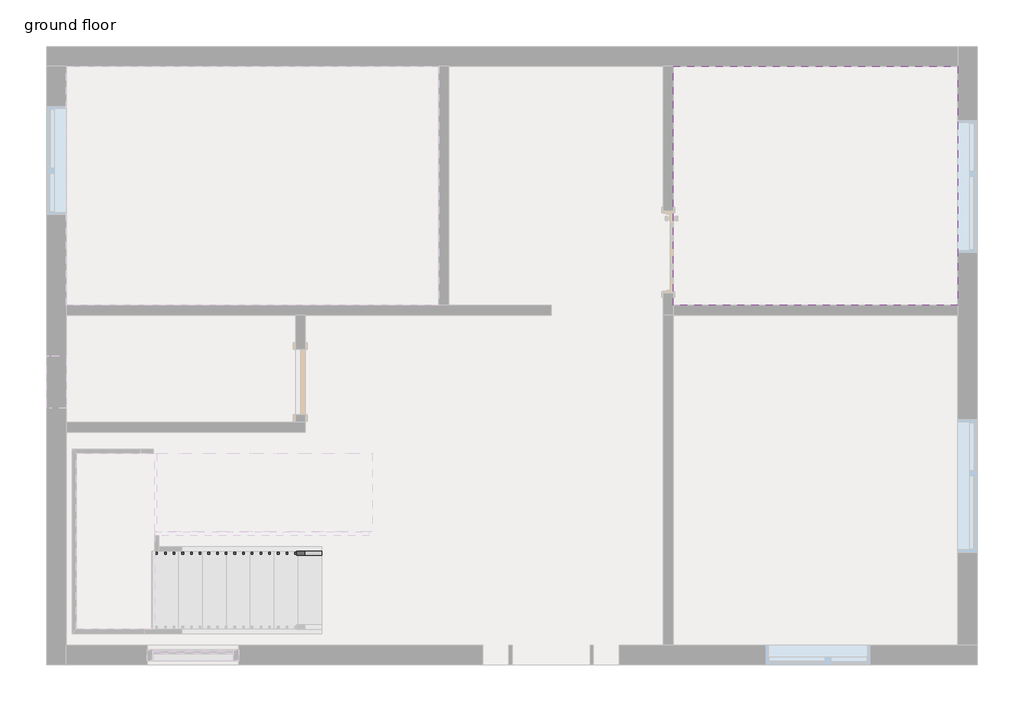
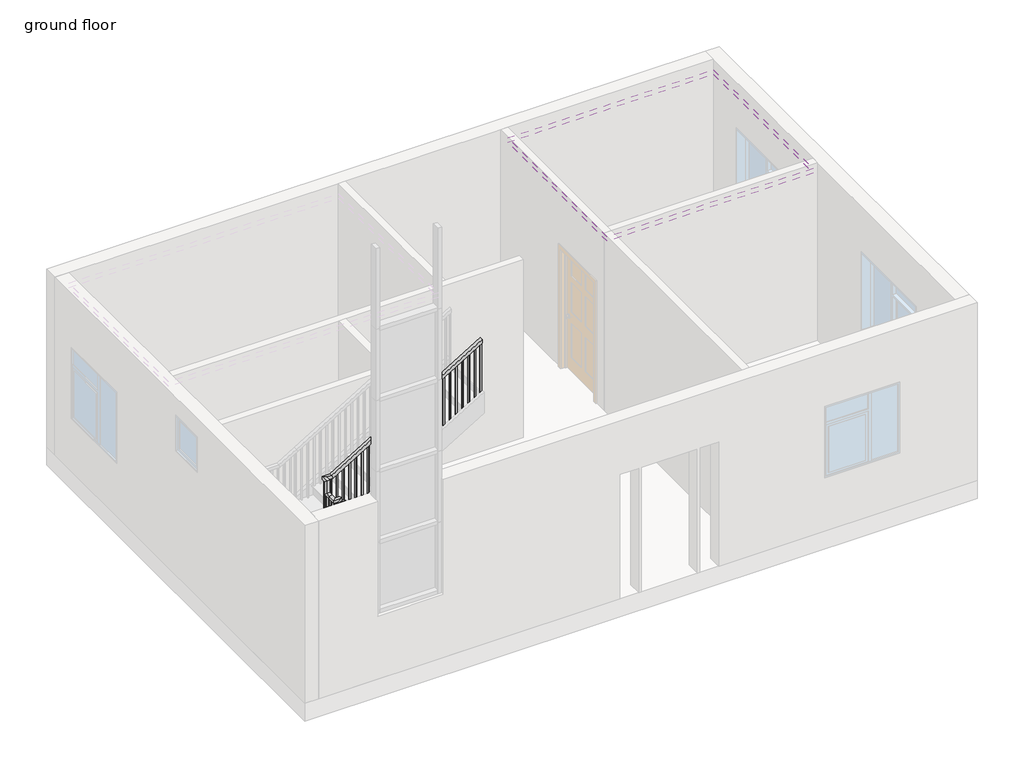
# One storey, part 2 of 3: 2 coverings, 1 railing.
"""IFC4 building model written with IfcOpenShell, lengths in millimetres."""

from ifc_helpers import new_model, si_unit, frame, origin, place, context, project, spatial, polyline, outline, extrude, faceted_brep, element, save

model = new_model("IFC4")

# Units and contexts
model_context = context("Model", 3, world=origin())
ifc_project = project(units=[si_unit("LENGTHUNIT", "METRE", prefix="MILLI")], contexts=[model_context])

# Site, building, storey
site = spatial("IfcSite", under=ifc_project)
building = spatial("IfcBuilding", under=site)
storey = spatial("IfcBuildingStorey", under=building, Name="ground floor", Elevation=304.8)

# Coverings
placement = place(None, origin())
element("IfcCovering", 1, ObjectType="METAL WHITE CEILING", at=placement, inside=storey, context=model_context, shape_type="SweptSolid", body=[
    extrude(outline(polyline([(-8505.3777023, 3436.0179075), (-8505.3777023, 6236.3679075), (-5171.6277023, 6236.3679075), (-5171.6277023, 3436.0179075), (-8505.3777023, 3436.0179075)])), frame((0.0, 0.0, 3175.0), z_axis=(0.0, 0.0, 1.0), x_axis=(1.0, 0.0, 0.0)), (0.0, 0.0, 1.0), 107.95),
])
element("IfcCovering", 2, ObjectType="METAL WHITE CEILING", at=placement, inside=storey, context=model_context, shape_type="SweptSolid", body=[
    extrude(outline(polyline([(-5171.6277023, 6236.3679075), (-5171.6277023, 3436.0179075), (-8505.3777023, 3436.0179075), (-8505.3777023, 6236.3679075), (-5171.6277023, 6236.3679075)]), holes=[polyline([(-5476.4277023, 5931.5679075), (-8200.5777023, 5931.5679075), (-8200.5777023, 3740.8179075), (-5476.4277023, 3740.8179075), (-5476.4277023, 5931.5679075)])]), frame((0.0, 0.0, 3098.8), z_axis=(0.0, 0.0, 1.0), x_axis=(1.0, 0.0, 0.0)), (0.0, 0.0, 1.0), 107.95),
    extrude(outline(polyline([(-7575.2115209, 5626.7679075), (-7575.2115209, 4045.6179075), (-7880.0115209, 4045.6179075), (-7880.0115209, 5626.7679075), (-7575.2115209, 5626.7679075)])), frame((0.0, 0.0, 3098.8), z_axis=(0.0, 0.0, 1.0), x_axis=(1.0, 0.0, 0.0)), (0.0, 0.0, 1.0), 107.95),
    extrude(outline(polyline([(-6965.6115209, 5626.7679075), (-6965.6115209, 4045.6179075), (-7270.4115209, 4045.6179075), (-7270.4115209, 5626.7679075), (-6965.6115209, 5626.7679075)])), frame((0.0, 0.0, 3098.8), z_axis=(0.0, 0.0, 1.0), x_axis=(1.0, 0.0, 0.0)), (0.0, 0.0, 1.0), 107.95),
    extrude(outline(polyline([(-6356.0115209, 5626.7679075), (-6356.0115209, 4045.6179075), (-6660.8115209, 4045.6179075), (-6660.8115209, 5626.7679075), (-6356.0115209, 5626.7679075)])), frame((0.0, 0.0, 3098.8), z_axis=(0.0, 0.0, 1.0), x_axis=(1.0, 0.0, 0.0)), (0.0, 0.0, 1.0), 107.95),
    extrude(outline(polyline([(-5746.4115209, 5626.7679075), (-5746.4115209, 4045.6179075), (-6051.2115209, 4045.6179075), (-6051.2115209, 5626.7679075), (-5746.4115209, 5626.7679075)])), frame((0.0, 0.0, 3098.8), z_axis=(0.0, 0.0, 1.0), x_axis=(1.0, 0.0, 0.0)), (0.0, 0.0, 1.0), 107.95),
])

# Railing
element("IfcRailing", 3, ObjectType="Handrail - Rectangular", at=placement, inside=storey, context=model_context, shape_type="SolidModel", body=[
    faceted_brep([(-12620.1777023, 508.6679075, 1388.5333333), (-12620.1777023, 508.6679075, 1329.1318731), (-12620.1777023, 559.4679075, 1329.1318731), (-12620.1777023, 559.4679075, 1388.5333333), (-14499.7777023, 508.6679075, 2527.6848485), (-14550.5777023, 508.6679075, 2499.071267), (-14550.5777023, 559.4679075, 2499.071267), (-14499.7777023, 559.4679075, 2527.6848485), (-14499.7777023, 508.6679075, 2573.8666667), (-14550.5777023, 508.6679075, 2523.0666667), (-14550.5777023, 559.4679075, 2523.0666667), (-14499.7777023, 559.4679075, 2573.8666667), (-14626.7777023, 508.6679075, 2573.8666667), (-14626.7777023, 508.6679075, 2523.0666667), (-14575.9777023, 559.4679075, 2523.0666667), (-14575.9777023, 559.4679075, 2573.8666667), (-14626.7777023, 635.6679075, 2573.8666667), (-14626.7777023, 635.6679075, 2523.0666667), (-14575.9777023, 635.6679075, 2523.0666667), (-14575.9777023, 635.6679075, 2573.8666667), (-14626.7777023, 711.8679075, 2573.8666667), (-14626.7777023, 762.6679075, 2523.0666667), (-14575.9777023, 762.6679075, 2523.0666667), (-14575.9777023, 711.8679075, 2573.8666667), (-14626.7777023, 711.8679075, 2789.3818182), (-14626.7777023, 762.6679075, 2738.5818182), (-14575.9777023, 762.6679075, 2738.5818182), (-14575.9777023, 711.8679075, 2789.3818182), (-14626.7777023, 838.8679075, 2789.3818182), (-14626.7777023, 838.8679075, 2738.5818182), (-14575.9777023, 788.0679075, 2738.5818182), (-14575.9777023, 788.0679075, 2789.3818182), (-14499.7777023, 838.8679075, 2789.3818182), (-14485.5852929, 838.8679075, 2738.5818182), (-14485.5852929, 788.0679075, 2738.5818182), (-14499.7777023, 788.0679075, 2789.3818182), (-12061.3777023, 838.8679075, 4267.2), (-12061.3777023, 788.0679075, 4267.2), (-12061.3777023, 788.0679075, 4207.7985397), (-12061.3777023, 838.8679075, 4207.7985397)], [[[0, 1, 2, 3]], [[1, 0, 4, 5]], [[2, 1, 5, 6]], [[3, 2, 6, 7]], [[0, 3, 7, 4]], [[5, 4, 8, 9]], [[6, 5, 9, 10]], [[7, 6, 10, 11]], [[4, 7, 11, 8]], [[9, 8, 12, 13]], [[10, 9, 13, 14]], [[11, 10, 14, 15]], [[8, 11, 15, 12]], [[13, 12, 16, 17]], [[14, 13, 17, 18]], [[15, 14, 18, 19]], [[12, 15, 19, 16]], [[17, 16, 20, 21]], [[18, 17, 21, 22]], [[19, 18, 22, 23]], [[16, 19, 23, 20]], [[21, 20, 24, 25]], [[22, 21, 25, 26]], [[23, 22, 26, 27]], [[20, 23, 27, 24]], [[25, 24, 28, 29]], [[26, 25, 29, 30]], [[27, 26, 30, 31]], [[24, 27, 31, 28]], [[29, 28, 32, 33]], [[30, 29, 33, 34]], [[31, 30, 34, 35]], [[28, 31, 35, 32]], [[36, 37, 38, 39]], [[33, 32, 36, 39]], [[34, 33, 39, 38]], [[35, 34, 38, 37]], [[32, 35, 37, 36]]]),
    extrude(outline(polyline([(4151.9955094, -12153.4527023), (4140.4500549, -12172.5027023), (3183.4666667, -12172.5027023), (3183.4666667, -12153.4527023), (4151.9955094, -12153.4527023)])), frame((0.0, 803.9429075, 0.0), z_axis=(0.0, 1.0, 0.0), x_axis=(0.0, 0.0, 1.0)), (0.0, 0.0, 1.0), 19.05),
    extrude(outline(polyline([(4090.4197519, -12255.0527023), (4078.8742973, -12274.1027023), (3183.4666667, -12274.1027023), (3183.4666667, -12255.0527023), (4090.4197519, -12255.0527023)])), frame((0.0, 803.9429075, 0.0), z_axis=(0.0, 1.0, 0.0), x_axis=(0.0, 0.0, 1.0)), (0.0, 0.0, 1.0), 19.05),
    extrude(outline(polyline([(4028.8439943, -12356.6527023), (4017.2985397, -12375.7027023), (3014.1333333, -12375.7027023), (3014.1333333, -12356.6527023), (4028.8439943, -12356.6527023)])), frame((0.0, 803.9429075, 0.0), z_axis=(0.0, 1.0, 0.0), x_axis=(0.0, 0.0, 1.0)), (0.0, 0.0, 1.0), 19.05),
    extrude(outline(polyline([(3967.2682367, -12458.2527023), (3955.7227822, -12477.3027023), (3014.1333333, -12477.3027023), (3014.1333333, -12458.2527023), (3967.2682367, -12458.2527023)])), frame((0.0, 803.9429075, 0.0), z_axis=(0.0, 1.0, 0.0), x_axis=(0.0, 0.0, 1.0)), (0.0, 0.0, 1.0), 19.05),
    extrude(outline(polyline([(3905.6924791, -12559.8527023), (3894.1470246, -12578.9027023), (3014.1333333, -12578.9027023), (3014.1333333, -12559.8527023), (3905.6924791, -12559.8527023)])), frame((0.0, 803.9429075, 0.0), z_axis=(0.0, 1.0, 0.0), x_axis=(0.0, 0.0, 1.0)), (0.0, 0.0, 1.0), 19.05),
    extrude(outline(polyline([(3844.1167216, -12661.4527023), (3832.571267, -12680.5027023), (2844.8, -12680.5027023), (2844.8, -12661.4527023), (3844.1167216, -12661.4527023)])), frame((0.0, 803.9429075, 0.0), z_axis=(0.0, 1.0, 0.0), x_axis=(0.0, 0.0, 1.0)), (0.0, 0.0, 1.0), 19.05),
    extrude(outline(polyline([(3782.540964, -12763.0527023), (3770.9955094, -12782.1027023), (2844.8, -12782.1027023), (2844.8, -12763.0527023), (3782.540964, -12763.0527023)])), frame((0.0, 803.9429075, 0.0), z_axis=(0.0, 1.0, 0.0), x_axis=(0.0, 0.0, 1.0)), (0.0, 0.0, 1.0), 19.05),
    extrude(outline(polyline([(3720.9652064, -12864.6527023), (3709.4197519, -12883.7027023), (2844.8, -12883.7027023), (2844.8, -12864.6527023), (3720.9652064, -12864.6527023)])), frame((0.0, 803.9429075, 0.0), z_axis=(0.0, 1.0, 0.0), x_axis=(0.0, 0.0, 1.0)), (0.0, 0.0, 1.0), 19.05),
    extrude(outline(polyline([(3659.3894488, -12966.2527023), (3647.8439943, -12985.3027023), (2675.4666667, -12985.3027023), (2675.4666667, -12966.2527023), (3659.3894488, -12966.2527023)])), frame((0.0, 803.9429075, 0.0), z_axis=(0.0, 1.0, 0.0), x_axis=(0.0, 0.0, 1.0)), (0.0, 0.0, 1.0), 19.05),
    extrude(outline(polyline([(3597.8136913, -13067.8527023), (3586.2682367, -13086.9027023), (2675.4666667, -13086.9027023), (2675.4666667, -13067.8527023), (3597.8136913, -13067.8527023)])), frame((0.0, 803.9429075, 0.0), z_axis=(0.0, 1.0, 0.0), x_axis=(0.0, 0.0, 1.0)), (0.0, 0.0, 1.0), 19.05),
    extrude(outline(polyline([(3536.2379337, -13169.4527023), (3524.6924791, -13188.5027023), (2675.4666667, -13188.5027023), (2675.4666667, -13169.4527023), (3536.2379337, -13169.4527023)])), frame((0.0, 803.9429075, 0.0), z_axis=(0.0, 1.0, 0.0), x_axis=(0.0, 0.0, 1.0)), (0.0, 0.0, 1.0), 19.05),
    extrude(outline(polyline([(3474.6621761, -13271.0527023), (3463.1167216, -13290.1027023), (2506.1333333, -13290.1027023), (2506.1333333, -13271.0527023), (3474.6621761, -13271.0527023)])), frame((0.0, 803.9429075, 0.0), z_axis=(0.0, 1.0, 0.0), x_axis=(0.0, 0.0, 1.0)), (0.0, 0.0, 1.0), 19.05),
    extrude(outline(polyline([(3413.0864185, -13372.6527023), (3401.540964, -13391.7027023), (2506.1333333, -13391.7027023), (2506.1333333, -13372.6527023), (3413.0864185, -13372.6527023)])), frame((0.0, 803.9429075, 0.0), z_axis=(0.0, 1.0, 0.0), x_axis=(0.0, 0.0, 1.0)), (0.0, 0.0, 1.0), 19.05),
    extrude(outline(polyline([(3351.510661, -13474.2527023), (3339.9652064, -13493.3027023), (2336.8, -13493.3027023), (2336.8, -13474.2527023), (3351.510661, -13474.2527023)])), frame((0.0, 803.9429075, 0.0), z_axis=(0.0, 1.0, 0.0), x_axis=(0.0, 0.0, 1.0)), (0.0, 0.0, 1.0), 19.05),
    extrude(outline(polyline([(3289.9349034, -13575.8527023), (3278.3894488, -13594.9027023), (2336.8, -13594.9027023), (2336.8, -13575.8527023), (3289.9349034, -13575.8527023)])), frame((0.0, 803.9429075, 0.0), z_axis=(0.0, 1.0, 0.0), x_axis=(0.0, 0.0, 1.0)), (0.0, 0.0, 1.0), 19.05),
    extrude(outline(polyline([(3228.3591458, -13677.4527023), (3216.8136913, -13696.5027023), (2336.8, -13696.5027023), (2336.8, -13677.4527023), (3228.3591458, -13677.4527023)])), frame((0.0, 803.9429075, 0.0), z_axis=(0.0, 1.0, 0.0), x_axis=(0.0, 0.0, 1.0)), (0.0, 0.0, 1.0), 19.05),
    extrude(outline(polyline([(3166.7833882, -13779.0527023), (3155.2379337, -13798.1027023), (2167.4666667, -13798.1027023), (2167.4666667, -13779.0527023), (3166.7833882, -13779.0527023)])), frame((0.0, 803.9429075, 0.0), z_axis=(0.0, 1.0, 0.0), x_axis=(0.0, 0.0, 1.0)), (0.0, 0.0, 1.0), 19.05),
    extrude(outline(polyline([(3105.2076307, -13880.6527023), (3093.6621761, -13899.7027023), (2167.4666667, -13899.7027023), (2167.4666667, -13880.6527023), (3105.2076307, -13880.6527023)])), frame((0.0, 803.9429075, 0.0), z_axis=(0.0, 1.0, 0.0), x_axis=(0.0, 0.0, 1.0)), (0.0, 0.0, 1.0), 19.05),
    extrude(outline(polyline([(3043.6318731, -13982.2527023), (3032.0864185, -14001.3027023), (2167.4666667, -14001.3027023), (2167.4666667, -13982.2527023), (3043.6318731, -13982.2527023)])), frame((0.0, 803.9429075, 0.0), z_axis=(0.0, 1.0, 0.0), x_axis=(0.0, 0.0, 1.0)), (0.0, 0.0, 1.0), 19.05),
    extrude(outline(polyline([(2982.0561155, -14083.8527023), (2970.510661, -14102.9027023), (1998.1333333, -14102.9027023), (1998.1333333, -14083.8527023), (2982.0561155, -14083.8527023)])), frame((0.0, 803.9429075, 0.0), z_axis=(0.0, 1.0, 0.0), x_axis=(0.0, 0.0, 1.0)), (0.0, 0.0, 1.0), 19.05),
    extrude(outline(polyline([(2920.4803579, -14185.4527023), (2908.9349034, -14204.5027023), (1998.1333333, -14204.5027023), (1998.1333333, -14185.4527023), (2920.4803579, -14185.4527023)])), frame((0.0, 803.9429075, 0.0), z_axis=(0.0, 1.0, 0.0), x_axis=(0.0, 0.0, 1.0)), (0.0, 0.0, 1.0), 19.05),
    extrude(outline(polyline([(2858.9046004, -14287.0527023), (2847.3591458, -14306.1027023), (1998.1333333, -14306.1027023), (1998.1333333, -14287.0527023), (2858.9046004, -14287.0527023)])), frame((0.0, 803.9429075, 0.0), z_axis=(0.0, 1.0, 0.0), x_axis=(0.0, 0.0, 1.0)), (0.0, 0.0, 1.0), 19.05),
    extrude(outline(polyline([(2797.3288428, -14388.6527023), (2785.7833882, -14407.7027023), (1828.8, -14407.7027023), (1828.8, -14388.6527023), (2797.3288428, -14388.6527023)])), frame((0.0, 803.9429075, 0.0), z_axis=(0.0, 1.0, 0.0), x_axis=(0.0, 0.0, 1.0)), (0.0, 0.0, 1.0), 19.05),
    extrude(outline(polyline([(2735.7530852, -14490.2527023), (2724.2076307, -14509.3027023), (1828.8, -14509.3027023), (1828.8, -14490.2527023), (2735.7530852, -14490.2527023)])), frame((0.0, 803.9429075, 0.0), z_axis=(0.0, 1.0, 0.0), x_axis=(0.0, 0.0, 1.0)), (0.0, 0.0, 1.0), 19.05),
    extrude(outline(polyline([(-14591.8527023, 727.7429075), (-14610.9027023, 727.7429075), (-14610.9027023, 746.7929075), (-14591.8527023, 746.7929075), (-14591.8527023, 727.7429075)])), frame((0.0, 0.0, 1659.4666667), z_axis=(0.0, 0.0, 1.0), x_axis=(1.0, 0.0, 0.0)), (0.0, 0.0, 1.0), 1079.1151515),
    extrude(outline(polyline([(-14591.8527023, 626.1429075), (-14610.9027023, 626.1429075), (-14610.9027023, 645.1929075), (-14591.8527023, 645.1929075), (-14591.8527023, 626.1429075)])), frame((0.0, 0.0, 1659.4666667), z_axis=(0.0, 0.0, 1.0), x_axis=(1.0, 0.0, 0.0)), (0.0, 0.0, 1.0), 863.6),
    extrude(outline(polyline([(-14541.0527023, 543.5929075), (-14541.0527023, 524.5429075), (-14560.1027023, 524.5429075), (-14560.1027023, 543.5929075), (-14541.0527023, 543.5929075)])), frame((0.0, 0.0, 1490.1333333), z_axis=(0.0, 0.0, 1.0), x_axis=(1.0, 0.0, 0.0)), (0.0, 0.0, 1.0), 1032.9333333),
    extrude(outline(polyline([(2431.7227822, -14439.4527023), (2443.2682367, -14458.5027023), (1490.1333333, -14458.5027023), (1490.1333333, -14439.4527023), (2431.7227822, -14439.4527023)])), frame((0.0, 524.5429075, 0.0), z_axis=(0.0, 1.0, 0.0), x_axis=(0.0, 0.0, 1.0)), (0.0, 0.0, 1.0), 19.05),
    extrude(outline(polyline([(2370.1470246, -14337.8527023), (2381.6924791, -14356.9027023), (1490.1333333, -14356.9027023), (1490.1333333, -14337.8527023), (2370.1470246, -14337.8527023)])), frame((0.0, 524.5429075, 0.0), z_axis=(0.0, 1.0, 0.0), x_axis=(0.0, 0.0, 1.0)), (0.0, 0.0, 1.0), 19.05),
    extrude(outline(polyline([(2308.571267, -14236.2527023), (2320.1167216, -14255.3027023), (1320.8, -14255.3027023), (1320.8, -14236.2527023), (2308.571267, -14236.2527023)])), frame((0.0, 524.5429075, 0.0), z_axis=(0.0, 1.0, 0.0), x_axis=(0.0, 0.0, 1.0)), (0.0, 0.0, 1.0), 19.05),
    extrude(outline(polyline([(2246.9955094, -14134.6527023), (2258.540964, -14153.7027023), (1320.8, -14153.7027023), (1320.8, -14134.6527023), (2246.9955094, -14134.6527023)])), frame((0.0, 524.5429075, 0.0), z_axis=(0.0, 1.0, 0.0), x_axis=(0.0, 0.0, 1.0)), (0.0, 0.0, 1.0), 19.05),
    extrude(outline(polyline([(2185.4197519, -14033.0527023), (2196.9652064, -14052.1027023), (1320.8, -14052.1027023), (1320.8, -14033.0527023), (2185.4197519, -14033.0527023)])), frame((0.0, 524.5429075, 0.0), z_axis=(0.0, 1.0, 0.0), x_axis=(0.0, 0.0, 1.0)), (0.0, 0.0, 1.0), 19.05),
    extrude(outline(polyline([(2123.8439943, -13931.4527023), (2135.3894488, -13950.5027023), (1151.4666667, -13950.5027023), (1151.4666667, -13931.4527023), (2123.8439943, -13931.4527023)])), frame((0.0, 524.5429075, 0.0), z_axis=(0.0, 1.0, 0.0), x_axis=(0.0, 0.0, 1.0)), (0.0, 0.0, 1.0), 19.05),
    extrude(outline(polyline([(2062.2682367, -13829.8527023), (2073.8136913, -13848.9027023), (1151.4666667, -13848.9027023), (1151.4666667, -13829.8527023), (2062.2682367, -13829.8527023)])), frame((0.0, 524.5429075, 0.0), z_axis=(0.0, 1.0, 0.0), x_axis=(0.0, 0.0, 1.0)), (0.0, 0.0, 1.0), 19.05),
    extrude(outline(polyline([(2000.6924791, -13728.2527023), (2012.2379337, -13747.3027023), (1151.4666667, -13747.3027023), (1151.4666667, -13728.2527023), (2000.6924791, -13728.2527023)])), frame((0.0, 524.5429075, 0.0), z_axis=(0.0, 1.0, 0.0), x_axis=(0.0, 0.0, 1.0)), (0.0, 0.0, 1.0), 19.05),
    extrude(outline(polyline([(1939.1167216, -13626.6527023), (1950.6621761, -13645.7027023), (982.1333333, -13645.7027023), (982.1333333, -13626.6527023), (1939.1167216, -13626.6527023)])), frame((0.0, 524.5429075, 0.0), z_axis=(0.0, 1.0, 0.0), x_axis=(0.0, 0.0, 1.0)), (0.0, 0.0, 1.0), 19.05),
    extrude(outline(polyline([(1877.540964, -13525.0527023), (1889.0864185, -13544.1027023), (982.1333333, -13544.1027023), (982.1333333, -13525.0527023), (1877.540964, -13525.0527023)])), frame((0.0, 524.5429075, 0.0), z_axis=(0.0, 1.0, 0.0), x_axis=(0.0, 0.0, 1.0)), (0.0, 0.0, 1.0), 19.05),
    extrude(outline(polyline([(1815.9652064, -13423.4527023), (1827.510661, -13442.5027023), (812.8, -13442.5027023), (812.8, -13423.4527023), (1815.9652064, -13423.4527023)])), frame((0.0, 524.5429075, 0.0), z_axis=(0.0, 1.0, 0.0), x_axis=(0.0, 0.0, 1.0)), (0.0, 0.0, 1.0), 19.05),
    extrude(outline(polyline([(1754.3894488, -13321.8527023), (1765.9349034, -13340.9027023), (812.8, -13340.9027023), (812.8, -13321.8527023), (1754.3894488, -13321.8527023)])), frame((0.0, 524.5429075, 0.0), z_axis=(0.0, 1.0, 0.0), x_axis=(0.0, 0.0, 1.0)), (0.0, 0.0, 1.0), 19.05),
    extrude(outline(polyline([(1692.8136913, -13220.2527023), (1704.3591458, -13239.3027023), (812.8, -13239.3027023), (812.8, -13220.2527023), (1692.8136913, -13220.2527023)])), frame((0.0, 524.5429075, 0.0), z_axis=(0.0, 1.0, 0.0), x_axis=(0.0, 0.0, 1.0)), (0.0, 0.0, 1.0), 19.05),
    extrude(outline(polyline([(1631.2379337, -13118.6527023), (1642.7833882, -13137.7027023), (643.4666667, -13137.7027023), (643.4666667, -13118.6527023), (1631.2379337, -13118.6527023)])), frame((0.0, 524.5429075, 0.0), z_axis=(0.0, 1.0, 0.0), x_axis=(0.0, 0.0, 1.0)), (0.0, 0.0, 1.0), 19.05),
    extrude(outline(polyline([(1569.6621761, -13017.0527023), (1581.2076307, -13036.1027023), (643.4666667, -13036.1027023), (643.4666667, -13017.0527023), (1569.6621761, -13017.0527023)])), frame((0.0, 524.5429075, 0.0), z_axis=(0.0, 1.0, 0.0), x_axis=(0.0, 0.0, 1.0)), (0.0, 0.0, 1.0), 19.05),
    extrude(outline(polyline([(1508.0864185, -12915.4527023), (1519.6318731, -12934.5027023), (643.4666667, -12934.5027023), (643.4666667, -12915.4527023), (1508.0864185, -12915.4527023)])), frame((0.0, 524.5429075, 0.0), z_axis=(0.0, 1.0, 0.0), x_axis=(0.0, 0.0, 1.0)), (0.0, 0.0, 1.0), 19.05),
    extrude(outline(polyline([(1446.510661, -12813.8527023), (1458.0561155, -12832.9027023), (474.1333333, -12832.9027023), (474.1333333, -12813.8527023), (1446.510661, -12813.8527023)])), frame((0.0, 524.5429075, 0.0), z_axis=(0.0, 1.0, 0.0), x_axis=(0.0, 0.0, 1.0)), (0.0, 0.0, 1.0), 19.05),
    extrude(outline(polyline([(1384.9349034, -12712.2527023), (1396.4803579, -12731.3027023), (474.1333333, -12731.3027023), (474.1333333, -12712.2527023), (1384.9349034, -12712.2527023)])), frame((0.0, 524.5429075, 0.0), z_axis=(0.0, 1.0, 0.0), x_axis=(0.0, 0.0, 1.0)), (0.0, 0.0, 1.0), 19.05),
    extrude(outline(polyline([(-14591.8527023, 803.9429075), (-14610.9027023, 803.9429075), (-14610.9027023, 822.9929075), (-14591.8527023, 822.9929075), (-14591.8527023, 803.9429075)])), frame((0.0, 0.0, 1659.4666667), z_axis=(0.0, 0.0, 1.0), x_axis=(1.0, 0.0, 0.0)), (0.0, 0.0, 1.0), 1079.1151515),
    extrude(outline(polyline([(-14591.8527023, 543.5929075), (-14591.8527023, 524.5429075), (-14610.9027023, 524.5429075), (-14610.9027023, 543.5929075), (-14591.8527023, 543.5929075)])), frame((0.0, 0.0, 1659.4666667), z_axis=(0.0, 0.0, 1.0), x_axis=(1.0, 0.0, 0.0)), (0.0, 0.0, 1.0), 863.6),
    extrude(outline(polyline([(4207.7985397, -12061.3777023), (4196.2530852, -12080.4277023), (3183.4666667, -12080.4277023), (3183.4666667, -12061.3777023), (4207.7985397, -12061.3777023)])), frame((0.0, 803.9429075, 0.0), z_axis=(0.0, 1.0, 0.0), x_axis=(0.0, 0.0, 1.0)), (0.0, 0.0, 1.0), 19.05),
    extrude(outline(polyline([(1329.1318731, -12620.1777023), (1340.6773276, -12639.2277023), (474.1333333, -12639.2277023), (474.1333333, -12620.1777023), (1329.1318731, -12620.1777023)])), frame((0.0, 524.5429075, 0.0), z_axis=(0.0, 1.0, 0.0), x_axis=(0.0, 0.0, 1.0)), (0.0, 0.0, 1.0), 19.05),
])

save(model, "model.ifc")

# Revit data of these elements
# Type "METAL WHITE CEILING"
#   Assembly Code = "C3030220"
#   built-in parameter 1002203 = 1 (stored number, unit not read)
#   built-in parameter 1002202 = 1 (stored number, unit not read)
#   Layers, outside or top first: 0' - 3 5/8" "Metal Stud Layer" (function 1); 0' - 0 5/8" "Laminate, Ivory, Matte" (function 5)
# Type "Handrail - Rectangular"
#   Assembly Code = "C2010400"
#   built-in parameter 1008612 = 0.0416667 (stored number, unit not read)
#   built-in parameter 1008611 = 0.0416667 (stored number, unit not read)
#   built-in parameter 1008609 = 0.333333 (stored number, unit not read)
#   built-in parameter 1008604 = 0.166667 (stored number, unit not read)
#   built-in parameter 1008603 = 0.166667 (stored number, unit not read)
#   Railing Height = 3' - 0"
#   built-in parameter 1008630 = 2
#   built-in parameter 1008610 = 2
#   built-in parameter 1008618 = Baluster - Square : 3/4"
# Element 1 (IfcCovering, "METAL WHITE CEILING")
#   Height Offset From Level = 9' - 5"
#   Phase Created = New Construction
#   Materials on its faces: "Laminate, Ivory, Matte", "Metal Stud Layer"
# Element 2 (IfcCovering, "METAL WHITE CEILING")
#   Height Offset From Level = 9' - 2"
#   Phase Created = New Construction
#   Materials on its faces: "Laminate, Ivory, Matte", "Metal Stud Layer"
# Element 3 (IfcRailing, "Handrail - Rectangular")
#   Phase Created = New Construction
# Materials
#   "Metal Stud Layer": class "Metal", colour RGB 199 199 199, transparency 0, Description = "Light gauge steel framing, thermal air layer", Cost = 0
#   "Laminate, Ivory, Matte": class "Plastic", colour RGB 247 247 239, transparency 0, Description = "Plastic Laminate - Ivory, Matte", Cost = 0
